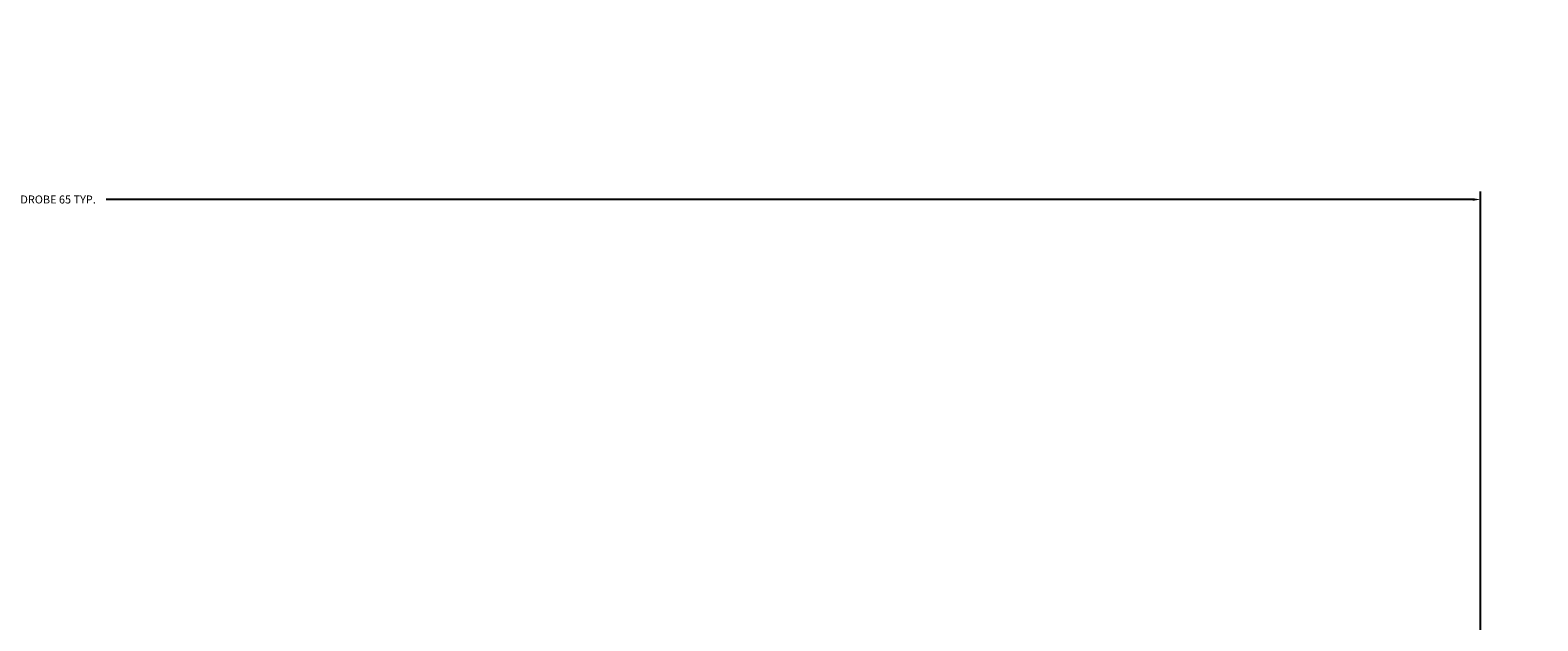
# Model space of a CAD drawing. Units: millimetres. Extents: x 27017497 to 27018854, y 7058029 to 7059154.
# Tile 41 of 91: x 27017655 to 27017689, y 7058459 to 7058472. Entities that reach past the tile are written whole.
import ezdxf

# ---------------------------------------------------------------- set-up
doc = ezdxf.new("R2010")
doc.units = ezdxf.units.MM
doc.layers.add('A-ANNO-DIMS', color=2, linetype='Continuous', lineweight=18)
doc.styles.get("Standard").update_dxf_attribs({"font": 'arial.ttf'})
doc.dimstyles.get("Standard").update_dxf_attribs({"dimtxt": 0.18, "dimasz": 0.18, "dimexe": 0.18, "dimexo": 0.0625, "dimgap": 0.09, "dimtad": 0, "dimtih": 1, "dimtoh": 1, "dimdec": 4, "dimzin": 0, "dimdsep": 46, "dimtxsty": 'Standard', "dimcen": 0.09, "dimadec": 0, "dimazin": 0, "dimtfac": 1, "dimtdec": 4, "dimtofl": 0, "dimtmove": 0, "dimatfit": 3, "dimfxl": 1, "dimtolj": 1, "dimtzin": 0, "dimarcsym": 0})

# ---------------------------------------------------------------- blocks, each defined once
blk = doc.blocks.new('*D45')
at = {"layer": 'A-ANNO-DIMS', "color": 0, "lineweight": -2, "transparency": 16777216}
for p, q in [((27017622.665, 7058458.704), (27017622.665, 7058468.604)), ((27017687.877, 7058458.704), (27017687.877, 7058468.604)), ((27017622.845, 7058468.424), (27017653.586, 7058468.424)), ((27017687.697, 7058468.424), (27017656.955, 7058468.424))]:
    blk.add_line(p, q, dxfattribs=at)
at = {"layer": 'A-ANNO-DIMS', "color": 0, "transparency": 16777216}
for points in [[(27017622.845, 7058468.454), (27017622.845, 7058468.394), (27017622.665, 7058468.424)], [(27017687.697, 7058468.454), (27017687.697, 7058468.394), (27017687.877, 7058468.424)]]:
    blk.add_solid(points, dxfattribs=at)
at = {"layer": 'Defpoints', "color": 0, "transparency": 16777216}
for p in [(27017687.877, 7058468.424), (27017622.665, 7058458.642), (27017687.877, 7058458.642)]:
    blk.add_point(p, dxfattribs=at)
at = {"layer": 'A-ANNO-DIMS', "color": 0, "transparency": 16777216, "insert": (27017655.271, 7058468.424), "char_height": 0.18, "attachment_point": 5}
blk.add_mtext('\\A1;WALL WARDROBE 65 TYP.', dxfattribs=at)
blk = doc.blocks.new('*D48')
at = {"layer": 'A-ANNO-DIMS', "color": 0, "lineweight": -2, "transparency": 16777216}
for p, q in [((27018463.498, 7058622.912), (27017497.536, 7058622.912)), ((27017497.716, 7058622.732), (27017497.716, 7058357.753)), ((27017497.716, 7058092.41), (27017497.716, 7058357.389)), ((27018555.129, 7058092.23), (27017497.536, 7058092.23))]:
    blk.add_line(p, q, dxfattribs=at)
at = {"layer": 'A-ANNO-DIMS', "color": 0, "transparency": 16777216}
for points in [[(27017497.686, 7058622.732), (27017497.746, 7058622.732), (27017497.716, 7058622.912)], [(27017497.686, 7058092.41), (27017497.746, 7058092.41), (27017497.716, 7058092.23)]]:
    blk.add_solid(points, dxfattribs=at)
at = {"layer": 'Defpoints', "color": 0, "transparency": 16777216}
for p in [(27018463.561, 7058622.912), (27017497.716, 7058092.23), (27018555.192, 7058092.23)]:
    blk.add_point(p, dxfattribs=at)
at = {"layer": 'A-ANNO-DIMS', "color": 0, "transparency": 16777216, "insert": (27017497.716, 7058357.571), "char_height": 0.18, "attachment_point": 5}
blk.add_mtext('\\A1;530.7', dxfattribs=at)

msp = doc.modelspace()

# ---------------------------------------------------------------- dimensions: what is measured, and where the dimension line sits
at = {"layer": 'A-ANNO-DIMS'}
dim = msp.add_linear_dim(base=(27017497.716, 7058092.23), p1=(27018463.561, 7058622.912), p2=(27018555.192, 7058092.23), angle=90, dimstyle='Standard', override={"dimdec": 1, "dimlfac": 1, "dimrnd": 0, "dimzin": 0, "dimdsep": 46, "dimlunit": 2}, dxfattribs=at)
dim.commit()
dim.dimension.update_dxf_attribs({"geometry": '*D48', "text_midpoint": (27017497.716, 7058357.571)})
dim = msp.add_linear_dim(base=(27017687.877, 7058468.424), p1=(27017622.665, 7058458.642), p2=(27017687.877, 7058458.642), text='WALL WARDROBE <> TYP.', dimstyle='Standard', override={"dimdec": 0, "dimlfac": 1, "dimrnd": 0, "dimzin": 0, "dimdsep": 46, "dimlunit": 2}, dxfattribs=at)
dim.commit()
dim.dimension.update_dxf_attribs({"geometry": '*D45', "text_midpoint": (27017655.271, 7058468.424)})

doc.saveas('drawing.dxf')
